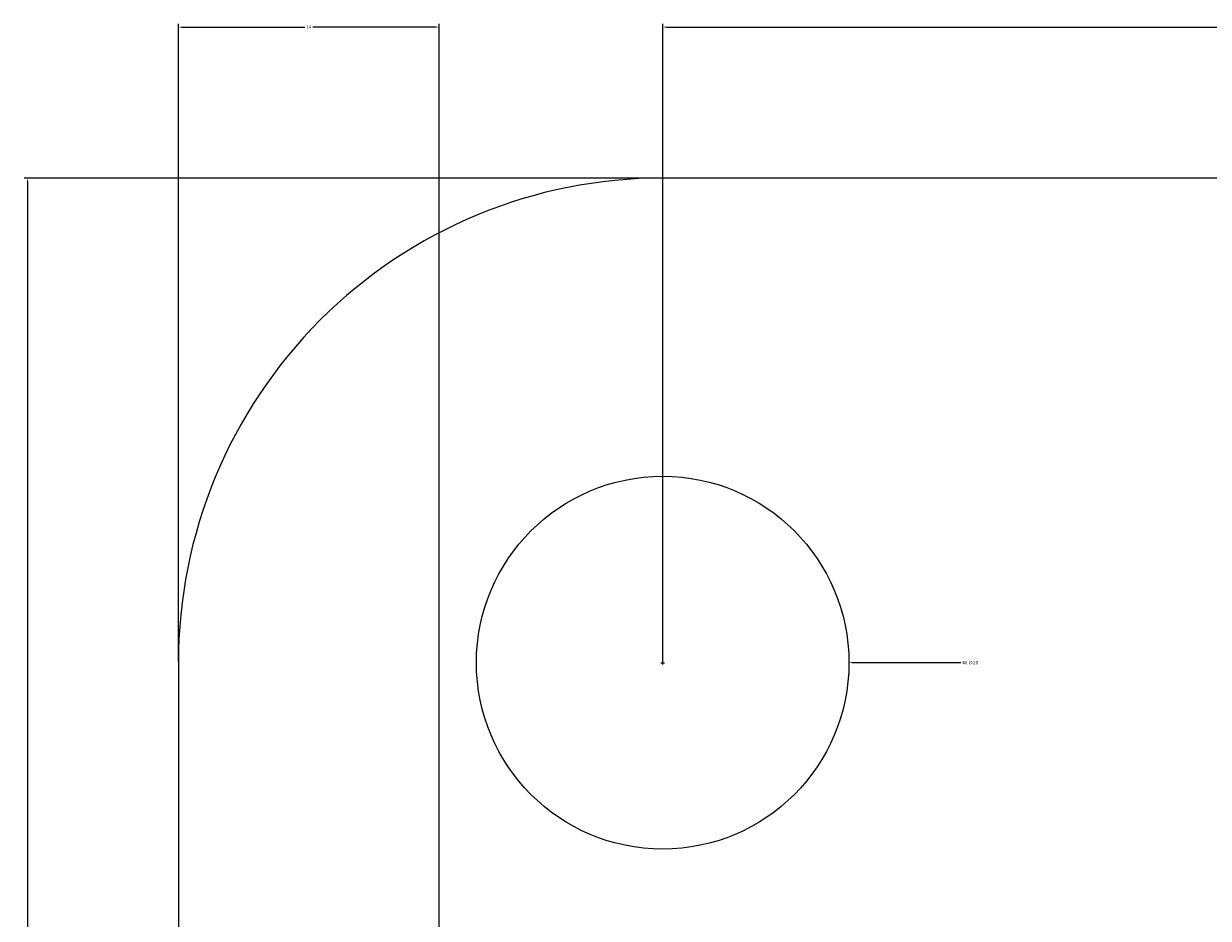
# Model space of a CAD drawing. Units: millimetres. Extents: x 2597 to 2768, y 1809 to 1980.
# Tile 3 of 7: x 2597 to 2661, y 1932 to 1980. Entities that reach past the tile are written whole.
import ezdxf

# ---------------------------------------------------------------- set-up
doc = ezdxf.new("R2010")
doc.units = ezdxf.units.MM
doc.layers.add('M-CONS', color=8, linetype='Continuous', lineweight=18)
doc.layers.add('M-DIMS', color=2, linetype='Continuous', lineweight=18)
doc.styles.get("Standard").update_dxf_attribs({"font": 'arial.ttf'})
doc.dimstyles.get("Standard").update_dxf_attribs({"dimtxt": 0.18, "dimasz": 0.18, "dimexe": 0.18, "dimexo": 0.0625, "dimgap": 0.09, "dimtad": 0, "dimtih": 1, "dimtoh": 1, "dimdec": 4, "dimzin": 0, "dimdsep": 46, "dimtxsty": 'Standard', "dimcen": 0.09, "dimadec": 0, "dimazin": 0, "dimtfac": 1, "dimtdec": 4, "dimtofl": 0, "dimtmove": 0, "dimatfit": 3, "dimfxl": 1, "dimtolj": 1, "dimtzin": 0, "dimarcsym": 0})

# ---------------------------------------------------------------- blocks, each defined once
blk = doc.blocks.new('*D4')
at = {"layer": 'Defpoints', "color": 0, "transparency": 16777216}
for p in [(2597.676, 1971.43), (2631.776, 1971.43), (2631.776, 1817.43)]:
    blk.add_point(p, dxfattribs=at)
at = {"layer": 'M-DIMS', "color": 0, "lineweight": -2, "transparency": 16777216}
for p, q in [((2631.713, 1971.43), (2597.496, 1971.43)), ((2597.676, 1971.25), (2597.676, 1894.612)), ((2597.676, 1817.61), (2597.676, 1894.248)), ((2631.713, 1817.43), (2597.496, 1817.43))]:
    blk.add_line(p, q, dxfattribs=at)
at = {"layer": 'M-DIMS', "color": 0, "transparency": 16777216}
for points in [[(2597.646, 1971.25), (2597.706, 1971.25), (2597.676, 1971.43)], [(2597.646, 1817.61), (2597.706, 1817.61), (2597.676, 1817.43)]]:
    blk.add_solid(points, dxfattribs=at)
at = {"layer": 'M-DIMS', "color": 0, "transparency": 16777216, "insert": (2597.676, 1894.43), "char_height": 0.18, "attachment_point": 5}
blk.add_mtext('\\A1;154', dxfattribs=at)
blk = doc.blocks.new('*D5')
at = {"layer": 'Defpoints', "color": 0, "transparency": 16777216}
for p in [(2733.776, 1979.53), (2631.776, 1945.43), (2733.776, 1945.43)]:
    blk.add_point(p, dxfattribs=at)
at = {"layer": 'M-DIMS', "color": 0, "lineweight": -2, "transparency": 16777216}
for p, q in [((2631.776, 1945.493), (2631.776, 1979.71)), ((2631.956, 1979.53), (2682.496, 1979.53)), ((2733.596, 1979.53), (2683.055, 1979.53)), ((2733.776, 1945.493), (2733.776, 1979.71))]:
    blk.add_line(p, q, dxfattribs=at)
at = {"layer": 'M-DIMS', "color": 0, "transparency": 16777216}
for points in [[(2631.956, 1979.56), (2631.956, 1979.5), (2631.776, 1979.53)], [(2733.596, 1979.56), (2733.596, 1979.5), (2733.776, 1979.53)]]:
    blk.add_solid(points, dxfattribs=at)
at = {"layer": 'M-DIMS', "color": 0, "transparency": 16777216, "insert": (2682.776, 1979.53), "char_height": 0.18, "attachment_point": 5}
blk.add_mtext('\\A1;102', dxfattribs=at)
blk = doc.blocks.new('*D8')
at = {"layer": 'Defpoints', "color": 0, "transparency": 16777216}
for p in [(2619.776, 1979.53), (2605.776, 1945.43), (2619.776, 1913.43)]:
    blk.add_point(p, dxfattribs=at)
at = {"layer": 'M-DIMS', "color": 0, "lineweight": -2, "transparency": 16777216}
for p, q in [((2605.776, 1945.493), (2605.776, 1979.71)), ((2605.956, 1979.53), (2612.565, 1979.53)), ((2619.596, 1979.53), (2612.986, 1979.53)), ((2619.776, 1913.493), (2619.776, 1979.71))]:
    blk.add_line(p, q, dxfattribs=at)
at = {"layer": 'M-DIMS', "color": 0, "transparency": 16777216}
for points in [[(2605.956, 1979.56), (2605.956, 1979.5), (2605.776, 1979.53)], [(2619.596, 1979.56), (2619.596, 1979.5), (2619.776, 1979.53)]]:
    blk.add_solid(points, dxfattribs=at)
at = {"layer": 'M-DIMS', "color": 0, "transparency": 16777216, "insert": (2612.776, 1979.53), "char_height": 0.18, "attachment_point": 5}
blk.add_mtext('\\A1;14', dxfattribs=at)
blk = doc.blocks.new('*D14')
at = {"layer": 'Defpoints', "color": 0, "transparency": 16777216}
for p in [(2621.776, 1945.43), (2641.776, 1945.43)]:
    blk.add_point(p, dxfattribs=at)
at = {"layer": 'M-DIMS', "color": 0, "lineweight": -2, "transparency": 16777216}
for p, q in [((2631.776, 1945.34), (2631.776, 1945.52)), ((2631.686, 1945.43), (2631.866, 1945.43)), ((2647.776, 1945.43), (2641.956, 1945.43))]:
    blk.add_line(p, q, dxfattribs=at)
at = {"layer": 'M-DIMS', "color": 0, "transparency": 16777216}
blk.add_solid([(2641.956, 1945.46), (2641.956, 1945.4), (2641.776, 1945.43)], dxfattribs=at)
at = {"layer": 'M-DIMS', "color": 0, "transparency": 16777216, "insert": (2648.284, 1945.43), "char_height": 0.18, "attachment_point": 5}
blk.add_mtext('\\A1;4X ∅20', dxfattribs=at)

msp = doc.modelspace()

# ---------------------------------------------------------------- linework, layer by layer
at = {"layer": 'M-CONS'}
msp.add_lwpolyline([(2631.7756, 1817.4301), (2733.7756, 1817.4301, 0.4142136), (2759.7756, 1843.4301), (2759.7756, 1945.4301, 0.4142136), (2733.7756, 1971.4301), (2631.7756, 1971.4301, 0.4142136), (2605.7756, 1945.4301), (2605.7756, 1843.4301, 0.4142136)], format="xyb", close=True, dxfattribs=at)
msp.add_circle((2631.7756, 1945.4301), 10, dxfattribs=at)

# ---------------------------------------------------------------- dimensions: what is measured, and where the dimension line sits
at = {"layer": 'M-DIMS'}
for base, p1, p2, picture, middle in [((2619.7756, 1979.5301), (2605.7756, 1945.4301), (2619.7756, 1913.4301), '*D8', (2612.7756, 1979.5301)), ((2733.7756, 1979.5301), (2631.7756, 1945.4301), (2733.7756, 1945.4301), '*D5', (2682.7756, 1979.5301))]:
    dim = msp.add_linear_dim(base=base, p1=p1, p2=p2, dimstyle='Standard', override={"dimdec": 0, "dimlfac": 1, "dimrnd": 0, "dimzin": 0, "dimdsep": 46, "dimlunit": 2}, dxfattribs=at)
    dim.commit()
    dim.dimension.update_dxf_attribs({"geometry": picture, "text_midpoint": middle})
dim = msp.add_linear_dim(base=(2597.6756, 1971.4301), p1=(2631.7756, 1817.4301), p2=(2631.7756, 1971.4301), angle=90, dimstyle='Standard', override={"dimdec": 0, "dimlfac": 1, "dimrnd": 0, "dimzin": 0, "dimdsep": 46, "dimlunit": 2}, dxfattribs=at)
dim.commit()
dim.dimension.update_dxf_attribs({"geometry": '*D4', "text_midpoint": (2597.6756, 1894.4301)})
dim = msp.add_diameter_dim_2p(p1=(2621.7756, 1945.4302), p2=(2641.7756, 1945.43), text='4X <>', dimstyle='Standard', override={"dimdec": 0, "dimlfac": 1, "dimrnd": 0, "dimzin": 0, "dimdsep": 46, "dimlunit": 2}, dxfattribs=at)
dim.commit()
dim.dimension.update_dxf_attribs({"geometry": '*D14', "text_midpoint": (2647.7756, 1945.4299), "dimtype": 163})

doc.saveas('drawing.dxf')
